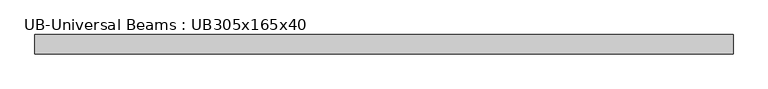
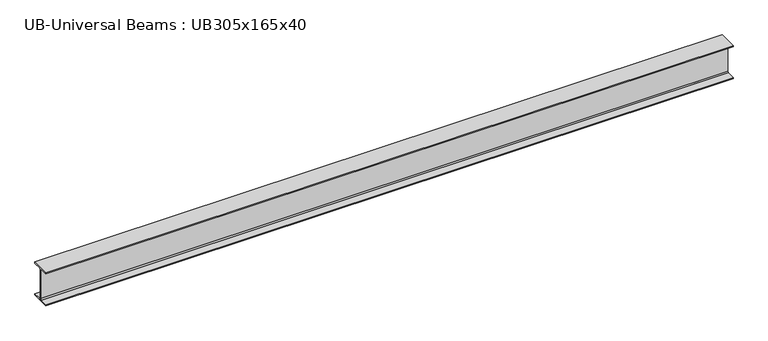
"""IFC4 building model written with IfcOpenShell, lengths in millimetres: beam geometry, UB-Universal Beams : UB305x165x40."""

from ifc_helpers import new_model, si_unit, point, frame, frame_2d, origin, place, context, project, spatial, polyline, circle_curve, trimmed, segment, composite_curve, outline, extrude, source, transform, mapped, element, save


def ub_universal_beams_ub305x165x40_db4e7ae9(model_context):
    return source(origin(), model_context, "Body", "SweptSolid", [
        extrude(outline(composite_curve([segment(polyline([(82.5, -141.5), (82.5, -151.7), (-82.5, -151.7), (-82.5, -141.5), (-11.9, -141.5)]), True, "CONTINUOUS"), segment(trimmed(circle_curve(frame_2d((-11.9, -132.6)), 8.9), [point((-11.9, -141.5))], [point((-3.0, -132.6))], True, "CARTESIAN"), True, "CONTINUOUS"), segment(polyline([(-3.0, -132.6), (-3.0, 132.6)]), True, "CONTINUOUS"), segment(trimmed(circle_curve(frame_2d((-11.9, 132.6)), 8.9), [point((-3.0, 132.6))], [point((-11.9, 141.5))], True, "CARTESIAN"), True, "CONTINUOUS"), segment(polyline([(-11.9, 141.5), (-82.5, 141.5), (-82.5, 151.7), (82.5, 151.7), (82.5, 141.5), (11.9, 141.5)]), True, "CONTINUOUS"), segment(trimmed(circle_curve(frame_2d((11.9, 132.6)), 8.9), [point((11.9, 141.5))], [point((3.0, 132.6))], True, "CARTESIAN"), True, "CONTINUOUS"), segment(polyline([(3.0, 132.6), (3.0, -132.6)]), True, "CONTINUOUS"), segment(trimmed(circle_curve(frame_2d((11.9, -132.6)), 8.9), [point((3.0, -132.6))], [point((11.9, -141.5))], True, "CARTESIAN"), True, "CONTINUOUS"), segment(polyline([(11.9, -141.5), (82.5, -141.5)]), True, "CONTINUOUS")], self_intersect=False)), frame((-3009.95, 0.0, 0.0), z_axis=(1.0, 0.0, 0.0), x_axis=(0.0, 1.0, 0.0)), (0.0, 0.0, 1.0), 5988.1),
    ])


if __name__ == "__main__":
    model = new_model("IFC4")
    model_context = context("Model", 3, world=origin())
    ifc_project = project(units=[si_unit("LENGTHUNIT", "METRE", prefix="MILLI")], contexts=[model_context])
    site = spatial("IfcSite", under=ifc_project)
    building = spatial("IfcBuilding", under=site)
    placement = place(None, origin())
    ub_universal_beams_ub305x165x40_shape = ub_universal_beams_ub305x165x40_db4e7ae9(model_context)
    element("IfcBeam", 1, ObjectType="UB-Universal Beams : UB305x165x40", at=placement, inside=building, context=model_context, shape_type="MappedRepresentation", body=[
        mapped(ub_universal_beams_ub305x165x40_shape, transform((0.0, 0.0, 0.0), x_axis=(1.0, 0.0, 0.0), y_axis=(0.0, 1.0, 0.0), z_axis=(0.0, 0.0, 1.0))),
    ])
    save(model, "model.ifc")

# Revit data of these elements
# Type "UB-Universal Beams : UB305x165x40"
#   Section Name Key = "UB305X165X40"
#   Width = 16.5 cm
#   Web Thickness = 0.6 cm
#   Web Fillet = 0.89 cm
#   Warping Constant = 164000.0 cm⁶
#   Torsional Moment of Inertia = 14.70 cm⁴
#   Section Area = 51.3 cm²
#   Plastic Modulus weak axis = 142.0 cm³
#   Plastic Modulus strong axis = 623.0 cm³
#   Nominal Weight = 40.2999 kgf/m
#   Moment of Inertia weak axis = 764.00 cm⁴
#   Moment of Inertia strong axis = 8503.00 cm⁴
#   Height = 30.34 cm
#   Flange Thickness = 1.02 cm
#   Elastic Modulus weak axis = 92.6 cm³
#   Elastic Modulus strong axis = 560.0 cm³
#   Centroid Vertical = 15.17 cm
#   Centroid Horizontal = 8.25 cm
#   Bolt Spacing = 9.0 cm
#   Length [instance default] = 1500 mm
#   Structural Material [instance default] = Metal - Steel 43-275
#   Type Comments = ""
#   Assembly Code = ""
# Element 1 (IfcBeam, "UB-Universal Beams : UB305x165x40")
#   Materials on its faces: "Metal - Steel 43-275"
# Materials
#   "Metal - Steel 43-275": class "Metal", colour RGB 247 247 247, transparency 0, Cost = 0
